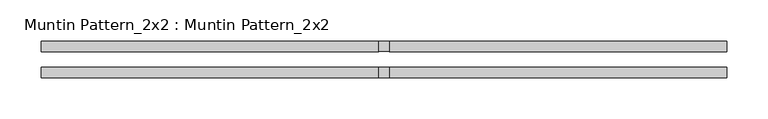
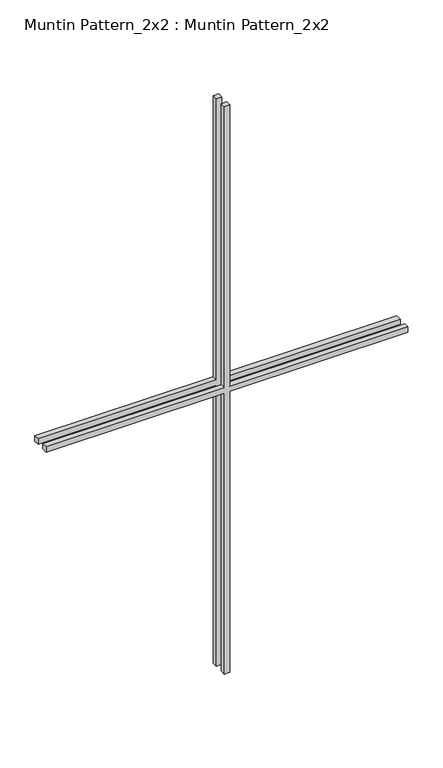
"""IFC4 building model written with IfcOpenShell, lengths in millimetres: proxy geometry, Muntin Pattern_2x2 : Muntin Pattern_2x2."""

from ifc_helpers import new_model, si_unit, frame, origin, place, context, project, spatial, polyline, outline, extrude, source, transform, mapped, element, save


def muntin_pattern_2x2_muntin_pattern_2x2_fa156a83(model_context):
    return source(origin(), model_context, "Body", "SweptSolid", [
        extrude(outline(polyline([(698.5, -6.35), (698.5, -417.6914087), (685.8, -417.6914087), (685.8, -6.35), (0.0, -6.35), (0.0, 6.35), (685.8, 6.35), (685.8, 417.6914087), (698.5, 417.6914087), (698.5, 6.35), (1384.3, 6.35), (1384.3, -6.35), (698.5, -6.35)])), frame((0.0, 9.525, 0.0), z_axis=(0.0, 1.0, 0.0), x_axis=(0.0, 0.0, 1.0)), (0.0, 0.0, 1.0), 12.7),
        extrude(outline(polyline([(698.5, -6.35), (698.5, -417.6914087), (685.8, -417.6914087), (685.8, -6.35), (0.0, -6.35), (0.0, 6.35), (685.8, 6.35), (685.8, 417.6914087), (698.5, 417.6914087), (698.5, 6.35), (1384.3, 6.35), (1384.3, -6.35), (698.5, -6.35)])), frame((0.0, -22.225, 0.0), z_axis=(0.0, 1.0, 0.0), x_axis=(0.0, 0.0, 1.0)), (0.0, 0.0, 1.0), 12.7),
    ])


if __name__ == "__main__":
    model = new_model("IFC4")
    model_context = context("Model", 3, world=origin())
    ifc_project = project(units=[si_unit("LENGTHUNIT", "METRE", prefix="MILLI")], contexts=[model_context])
    site = spatial("IfcSite", under=ifc_project)
    building = spatial("IfcBuilding", under=site)
    placement = place(None, origin())
    muntin_pattern_2x2_muntin_pattern_2x2_shape = muntin_pattern_2x2_muntin_pattern_2x2_fa156a83(model_context)
    element("IfcBuildingElementProxy", 1, Name="Muntin Pattern_2x2 : Muntin Pattern_2x2", ObjectType="Muntin Pattern_2x2 : Muntin Pattern_2x2", at=placement, inside=building, context=model_context, shape_type="MappedRepresentation", body=[
        mapped(muntin_pattern_2x2_muntin_pattern_2x2_shape, transform((0.0, 0.0, 0.0), x_axis=(1.0, 0.0, 0.0), y_axis=(0.0, 1.0, 0.0), z_axis=(0.0, 0.0, 1.0))),
    ])
    save(model, "model.ifc")

# Revit data of these elements
# Type "Muntin Pattern_2x2 : Muntin Pattern_2x2"
#   Width [instance default] = 4' - 0"
#   Thickness = 0' - 0 1/2"
#   Height [instance default] = 4' - 0"
#   Distance = 0' - 0 3/4"
#   Interior Material [instance default] = none
#   Exterior Material [instance default] = none
#   Default Elevation = 0
# Element 1 (IfcBuildingElementProxy, "Muntin Pattern_2x2 : Muntin Pattern_2x2")
#   Width = 2' - 8.88909"
#   Height = 4' - 6 1/2"
#   Interior Material = Wood - Stained
#   Exterior Material = Clad - White
#   Materials on its faces: "Clad - White", "Wood - Stained"
# Materials
#   "Clad - White": class "Wood", colour RGB 242 242 238, transparency 0, Cost = 0
#   "Wood - Stained": class "Wood", colour RGB 224 178 126, transparency 0, Cost = 0
